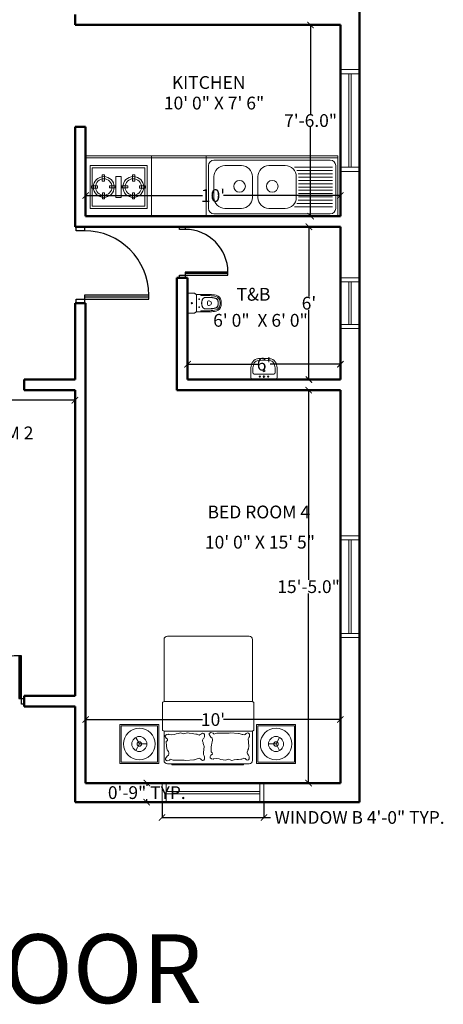
# Model space of a CAD drawing. Units: inches. Extents: x 147 to 1638, y 107 to 941.
# Tile 9 of 17: x 542 to 741, y 107 to 570. Entities that reach past the tile are written whole.
import ezdxf

# ---------------------------------------------------------------- set-up
doc = ezdxf.new("R2010")
doc.units = ezdxf.units.IN
doc.header["$MEASUREMENT"] = 0
for name, color, linetype, lineweight in [('A-ANNO-DIMS', 2, 'Continuous', 15), ('A-ANNO-TEXT', 7, 'Continuous', 25), ('A-AREA-IDEN', 7, 'Continuous', 18), ('A-Door', 150, 'Continuous', 25), ('A-EQPM', 8, 'Continuous', 18), ('A-FLOR-CASE', 9, 'Continuous', 20), ('A-FLOR-FIXT', 9, 'Continuous', 18), ('furniture', 50, 'Continuous', 18), ('walls', 7, 'Continuous', 50), ('windows', 3, 'Continuous', 20)]:
    doc.layers.add(name, color=color, linetype=linetype, lineweight=lineweight)
doc.layers.add('A-Glaz', color=92, linetype='Continuous')
doc.layers.add('NT', color=1, linetype='Continuous')
doc.styles.get("Standard").update_dxf_attribs({"font": 'arial.ttf'})
doc.dimstyles.get("Standard").update_dxf_attribs({"dimtxt": 6, "dimasz": 3, "dimexe": 0.18, "dimexo": 0.0625, "dimgap": 0.09, "dimtad": 0, "dimtih": 1, "dimtoh": 1, "dimdec": 1, "dimzin": 0, "dimdsep": 46, "dimlunit": 3, "dimtxsty": 'Standard', "dimblk": 'ARCHTICK', "dimcen": 0.09, "dimadec": 0, "dimazin": 0, "dimtfac": 1, "dimtdec": 1, "dimtofl": 0, "dimtmove": 0, "dimatfit": 3, "dimfxl": 1, "dimtolj": 1, "dimtzin": 0, "dimarcsym": 0})

# ---------------------------------------------------------------- blocks, each defined once
blk = doc.blocks.new('A$C087A3AA9')
at = {"layer": 'A-Door'}
for points in [[(853, 95), (853, 853), (805, 853), (805, 95)], [(47, 95), (47, 0), (0, 0), (0, 95)], [(900, 95), (900, 0), (853, 0), (853, 95)]]:
    blk.add_lwpolyline(points, close=True, dxfattribs=at)
at = {"layer": 'A-Glaz'}
blk.add_line((829, 853), (829, 95), dxfattribs=at)
at = {"layer": 'NT'}
blk.add_arc((805, 95), 758, 90, 180, dxfattribs=at)
blk = doc.blocks.new('_ArchTick')
at = {"color": 0, "linetype": 'ByBlock', "const_width": 0.15}
blk.add_lwpolyline([(-0.5, -0.5), (0.5, 0.5)], dxfattribs=at)
blk = doc.blocks.new('*D18')
at = {"layer": 'A-ANNO-DIMS', "color": 0, "lineweight": -2, "transparency": 16777216}
for p, q in [((620.94, 408.03), (620.94, 408.14)), ((692.94, 408.03), (692.94, 408.14)), ((620.94, 407.96), (654.08, 407.96)), ((692.94, 407.96), (659.81, 407.96))]:
    blk.add_line(p, q, dxfattribs=at)
at = {"layer": 'Defpoints', "color": 0, "lineweight": -2, "transparency": 16777216}
for p in [(620.94, 407.96), (692.94, 407.96), (692.94, 407.96)]:
    blk.add_point(p, dxfattribs=at)
at = {"layer": 'A-ANNO-DIMS', "color": 0, "lineweight": -2, "transparency": 16777216, "xscale": 3, "yscale": 3, "zscale": 3, "rotation": 180}
blk.add_blockref('_ArchTick', (620.94, 407.96), dxfattribs=at)
at = {"layer": 'A-ANNO-DIMS', "color": 0, "lineweight": -2, "transparency": 16777216, "xscale": 3, "yscale": 3, "zscale": 3}
blk.add_blockref('_ArchTick', (692.94, 407.96), dxfattribs=at)
at = {"layer": 'A-ANNO-DIMS', "color": 0, "transparency": 16777216, "insert": (656.94, 407.96), "char_height": 6, "attachment_point": 5}
blk.add_mtext("\\A1;6'", dxfattribs=at)
blk = doc.blocks.new('*D19')
at = {"layer": 'A-ANNO-DIMS', "color": 0, "lineweight": -2, "transparency": 16777216}
for p, q in [((678.55, 472.72), (677.93, 472.72)), ((678.11, 472.72), (678.11, 439.87)), ((678.11, 400.72), (678.11, 433.56)), ((678.55, 400.72), (677.93, 400.72))]:
    blk.add_line(p, q, dxfattribs=at)
at = {"layer": 'Defpoints', "color": 0, "lineweight": -2, "transparency": 16777216}
for p in [(678.61, 472.72), (678.11, 400.72), (678.61, 400.72)]:
    blk.add_point(p, dxfattribs=at)
at = {"layer": 'A-ANNO-DIMS', "color": 0, "lineweight": -2, "transparency": 16777216, "xscale": 3, "yscale": 3, "zscale": 3}
for p, rotation in [((678.11, 472.72), 90), ((678.11, 400.72), 270)]:
    blk.add_blockref('_ArchTick', p, dxfattribs=dict(at, rotation=rotation))
at = {"layer": 'A-ANNO-DIMS', "color": 0, "transparency": 16777216, "insert": (678.11, 436.72), "char_height": 6, "attachment_point": 5}
blk.add_mtext("\\A1;6'", dxfattribs=at)
blk = doc.blocks.new('*D20')
at = {"layer": 'A-ANNO-DIMS', "color": 0, "lineweight": -2, "transparency": 16777216}
for p, q in [((665.57, 567.72), (679.08, 567.72)), ((678.9, 567.72), (678.9, 525.87)), ((678.9, 477.72), (678.9, 519.56)), ((665.57, 477.72), (679.08, 477.72))]:
    blk.add_line(p, q, dxfattribs=at)
at = {"layer": 'Defpoints', "color": 0, "lineweight": -2, "transparency": 16777216}
for p in [(665.51, 567.72), (665.51, 477.72), (678.9, 477.72)]:
    blk.add_point(p, dxfattribs=at)
at = {"layer": 'A-ANNO-DIMS', "color": 0, "lineweight": -2, "transparency": 16777216, "xscale": 3, "yscale": 3, "zscale": 3}
for p, rotation in [((678.9, 567.72), 90), ((678.9, 477.72), 270)]:
    blk.add_blockref('_ArchTick', p, dxfattribs=dict(at, rotation=rotation))
at = {"layer": 'A-ANNO-DIMS', "color": 0, "transparency": 16777216, "insert": (678.9, 522.72), "char_height": 6, "attachment_point": 5}
blk.add_mtext('\\A1;7\'-6.0"', dxfattribs=at)
blk = doc.blocks.new('*D21')
at = {"layer": 'A-ANNO-DIMS', "color": 0, "lineweight": -2, "transparency": 16777216}
for p, q in [((572.94, 484.18), (572.94, 487.58)), ((572.94, 487.4), (628.05, 487.4)), ((692.94, 487.4), (637.84, 487.4)), ((692.94, 484.18), (692.94, 487.58))]:
    blk.add_line(p, q, dxfattribs=at)
at = {"layer": 'Defpoints', "color": 0, "lineweight": -2, "transparency": 16777216}
for p in [(692.94, 487.4), (572.94, 484.12), (692.94, 484.12)]:
    blk.add_point(p, dxfattribs=at)
at = {"layer": 'A-ANNO-DIMS', "color": 0, "lineweight": -2, "transparency": 16777216, "xscale": 3, "yscale": 3, "zscale": 3, "rotation": 180}
blk.add_blockref('_ArchTick', (572.94, 487.4), dxfattribs=at)
at = {"layer": 'A-ANNO-DIMS', "color": 0, "lineweight": -2, "transparency": 16777216, "xscale": 3, "yscale": 3, "zscale": 3}
blk.add_blockref('_ArchTick', (692.94, 487.4), dxfattribs=at)
at = {"layer": 'A-ANNO-DIMS', "color": 0, "transparency": 16777216, "insert": (632.94, 487.4), "char_height": 6, "attachment_point": 5}
blk.add_mtext("\\A1;10'", dxfattribs=at)
blk = doc.blocks.new('*D22')
at = {"layer": 'A-ANNO-DIMS', "color": 0, "lineweight": -2, "transparency": 16777216}
for p, q in [((572.94, 231.3), (572.94, 240.81)), ((572.94, 240.63), (628.05, 240.63)), ((692.94, 240.63), (637.84, 240.63)), ((692.94, 231.3), (692.94, 240.81))]:
    blk.add_line(p, q, dxfattribs=at)
at = {"layer": 'Defpoints', "color": 0, "lineweight": -2, "transparency": 16777216}
for p in [(692.94, 240.63), (572.94, 231.24), (692.94, 231.24)]:
    blk.add_point(p, dxfattribs=at)
at = {"layer": 'A-ANNO-DIMS', "color": 0, "lineweight": -2, "transparency": 16777216, "xscale": 3, "yscale": 3, "zscale": 3, "rotation": 180}
blk.add_blockref('_ArchTick', (572.94, 240.63), dxfattribs=at)
at = {"layer": 'A-ANNO-DIMS', "color": 0, "lineweight": -2, "transparency": 16777216, "xscale": 3, "yscale": 3, "zscale": 3}
blk.add_blockref('_ArchTick', (692.94, 240.63), dxfattribs=at)
at = {"layer": 'A-ANNO-DIMS', "color": 0, "transparency": 16777216, "insert": (632.94, 240.63), "char_height": 6, "attachment_point": 5}
blk.add_mtext("\\A1;10'", dxfattribs=at)
blk = doc.blocks.new('*D23')
at = {"layer": 'A-ANNO-DIMS', "color": 0, "lineweight": -2, "transparency": 16777216}
for p, q in [((684.27, 395.72), (677.76, 395.72)), ((677.94, 395.72), (677.94, 306.37)), ((677.94, 210.72), (677.94, 300.06)), ((684.27, 210.72), (677.76, 210.72))]:
    blk.add_line(p, q, dxfattribs=at)
at = {"layer": 'Defpoints', "color": 0, "lineweight": -2, "transparency": 16777216}
for p in [(684.33, 395.72), (677.94, 210.72), (684.33, 210.72)]:
    blk.add_point(p, dxfattribs=at)
at = {"layer": 'A-ANNO-DIMS', "color": 0, "lineweight": -2, "transparency": 16777216, "xscale": 3, "yscale": 3, "zscale": 3}
for p, rotation in [((677.94, 395.72), 90), ((677.94, 210.72), 270)]:
    blk.add_blockref('_ArchTick', p, dxfattribs=dict(at, rotation=rotation))
at = {"layer": 'A-ANNO-DIMS', "color": 0, "transparency": 16777216, "insert": (677.94, 303.22), "char_height": 6, "attachment_point": 5}
blk.add_mtext('\\A1;15\'-5.0"', dxfattribs=at)
blk = doc.blocks.new('*D29')
at = {"layer": 'A-ANNO-DIMS', "color": 0, "lineweight": -2, "transparency": 16777216}
for p, q in [((471.94, 391.04), (471.94, 391.15)), ((471.94, 390.97), (517.09, 390.97)), ((567.94, 390.97), (522.8, 390.97)), ((567.94, 391.04), (567.94, 391.15))]:
    blk.add_line(p, q, dxfattribs=at)
at = {"layer": 'Defpoints', "color": 0, "lineweight": -2, "transparency": 16777216}
for p in [(471.94, 390.97), (567.94, 390.97), (567.94, 390.97)]:
    blk.add_point(p, dxfattribs=at)
at = {"layer": 'A-ANNO-DIMS', "color": 0, "lineweight": -2, "transparency": 16777216, "xscale": 3, "yscale": 3, "zscale": 3, "rotation": 180}
blk.add_blockref('_ArchTick', (471.94, 390.97), dxfattribs=at)
at = {"layer": 'A-ANNO-DIMS', "color": 0, "lineweight": -2, "transparency": 16777216, "xscale": 3, "yscale": 3, "zscale": 3}
blk.add_blockref('_ArchTick', (567.94, 390.97), dxfattribs=at)
at = {"layer": 'A-ANNO-DIMS', "color": 0, "transparency": 16777216, "insert": (519.94, 390.97), "char_height": 6, "attachment_point": 5}
blk.add_mtext("\\A1;8'", dxfattribs=at)
blk = doc.blocks.new('MAT-P14')
for p, q in [((-1.337, 1.348), (-1.337, 1.948)), ((-1.337, 1.948), (-0.737, 1.948)), ((-1.317, 1.928), (-0.757, 1.928)), ((-1.317, 1.368), (-1.317, 1.928)), ((-0.757, 1.368), (-0.757, 1.928)), ((-0.737, 1.348), (-0.737, 1.948)), ((0.625, 1.95), (-0.625, 1.95)), ((0.753, 1.348), (0.753, 1.948)), ((1.353, 1.948), (0.753, 1.948)), ((1.333, 1.928), (0.773, 1.928)), ((0.773, 1.368), (0.773, 1.928)), ((1.333, 1.368), (1.333, 1.928)), ((1.353, 1.348), (1.353, 1.948)), ((-1.037, 1.648), (-1.091, 1.749)), ((1.053, 1.648), (1.108, 1.749)), ((-1.037, 1.648), (-1.091, 1.547)), ((-1.037, 1.648), (-0.922, 1.648)), ((1.053, 1.648), (0.938, 1.648)), ((1.053, 1.648), (1.108, 1.547)), ((-1.317, 1.368), (-0.757, 1.368)), ((1.333, 1.368), (0.773, 1.368)), ((-1.337, 1.348), (-0.737, 1.348)), ((1.353, 1.348), (0.753, 1.348))]:
    blk.add_line(p, q)
blk.add_lwpolyline([(-0.542, 1.95), (-0.542, 1.967), (0.558, 1.967), (0.558, 1.95)], close=True)
for points in [[(-0.675, 1.45), (-0.675, 1.9, -0.414214), (-0.625, 1.95), (0.625, 1.95, -0.414214), (0.675, 1.9), (0.675, 1.45)], [(-0.675, 1, -0.414214), (-0.7, 1.025), (-0.7, 1.425, -0.414214), (-0.675, 1.45), (0.675, 1.45, -0.414214), (0.7, 1.425), (0.7, 1.025, -0.414214), (0.675, 1)], [(-0.625, 0, -0.414214), (-0.675, 0.05), (-0.675, 1), (0.675, 1), (0.675, 0.05, -0.414214), (0.625, 0)]]:
    blk.add_lwpolyline(points, format="xyb", close=True)
for points in [[(-0.614, 1.818), (-0.626, 1.838), (-0.626, 1.877), (-0.614, 1.891), (-0.596, 1.896), (-0.579, 1.886), (-0.563, 1.872), (-0.545, 1.863), (-0.516, 1.879), (-0.497, 1.882), (-0.465, 1.884), (-0.439, 1.887), (-0.395, 1.892), (-0.363, 1.9), (-0.309, 1.882), (-0.262, 1.897), (-0.23, 1.892), (-0.192, 1.884), (-0.166, 1.873), (-0.128, 1.868), (-0.082, 1.875), (-0.076, 1.88), (-0.052, 1.875), (-0.028, 1.861), (-0.028, 1.841), (-0.04, 1.817), (-0.064, 1.802), (-0.06, 1.781), (-0.043, 1.768), (-0.046, 1.697), (-0.05, 1.662), (-0.056, 1.64), (-0.062, 1.612), (-0.068, 1.596), (-0.068, 1.579), (-0.063, 1.56), (-0.039, 1.545), (-0.015, 1.505), (-0.015, 1.486), (-0.038, 1.471), (-0.075, 1.482), (-0.081, 1.487), (-0.087, 1.497), (-0.134, 1.481), (-0.304, 1.482), (-0.318, 1.482), (-0.335, 1.479), (-0.464, 1.488), (-0.467, 1.486), (-0.473, 1.486), (-0.517, 1.503), (-0.53, 1.505), (-0.548, 1.51), (-0.566, 1.501), (-0.581, 1.487), (-0.599, 1.477), (-0.617, 1.482), (-0.629, 1.497), (-0.629, 1.536), (-0.623, 1.55), (-0.611, 1.57), (-0.614, 1.614), (-0.615, 1.627), (-0.618, 1.644), (-0.619, 1.66), (-0.62, 1.675), (-0.62, 1.695), (-0.618, 1.707), (-0.614, 1.723), (-0.608, 1.739), (-0.604, 1.75), (-0.598, 1.771), (-0.596, 1.785), (-0.6, 1.798), (-0.614, 1.819)], [(0.069, 1.559), (0.057, 1.54), (0.057, 1.501), (0.069, 1.486), (0.087, 1.481), (0.105, 1.491), (0.121, 1.505), (0.139, 1.514), (0.168, 1.498), (0.187, 1.496), (0.219, 1.493), (0.244, 1.49), (0.289, 1.485), (0.321, 1.477), (0.374, 1.495), (0.422, 1.48), (0.454, 1.486), (0.492, 1.493), (0.517, 1.504), (0.555, 1.509), (0.602, 1.502), (0.608, 1.497), (0.632, 1.502), (0.656, 1.517), (0.656, 1.536), (0.644, 1.561), (0.62, 1.575), (0.624, 1.596), (0.641, 1.609), (0.637, 1.68), (0.633, 1.715), (0.628, 1.738), (0.606, 1.765), (0.6, 1.781), (0.6, 1.798), (0.605, 1.817), (0.629, 1.832), (0.654, 1.872), (0.654, 1.892), (0.63, 1.906), (0.593, 1.895), (0.587, 1.891), (0.581, 1.881), (0.534, 1.896), (0.379, 1.896), (0.366, 1.896), (0.348, 1.898), (0.22, 1.89), (0.216, 1.891), (0.21, 1.891), (0.167, 1.875), (0.154, 1.872), (0.136, 1.867), (0.118, 1.876), (0.102, 1.89), (0.085, 1.9), (0.067, 1.895), (0.055, 1.881), (0.055, 1.842), (0.061, 1.827), (0.073, 1.807), (0.07, 1.764), (0.069, 1.75), (0.066, 1.733), (0.065, 1.718), (0.063, 1.703), (0.063, 1.682), (0.066, 1.67), (0.07, 1.655), (0.075, 1.638), (0.079, 1.627), (0.086, 1.607), (0.087, 1.592), (0.083, 1.579), (0.07, 1.559)]]:
    blk.add_lwpolyline(points)
for centre, radius in [((-1.037, 1.648), 0.24), ((1.053, 1.648), 0.24), ((-1.037, 1.648), 0.115), ((-1.037, 1.648), 0.035), ((1.053, 1.648), 0.115), ((1.053, 1.648), 0.035)]:
    blk.add_circle(centre, radius)
blk = doc.blocks.new('2SAINDA')
at = {"color": 0, "linetype": 'ByBlock'}
for p, q in [((0.018, 0.2), (0.141, 0.2)), ((0, 0.188), (0, -0.188)), ((0.157, 0.192), (0.162, 0.188)), ((0.18, -0.164), (0.18, 0.164)), ((0.279, 0.159), (0.261, 0.176)), ((0.437, 0.047), (0.424, 0.047)), ((0.157, -0.192), (0.162, -0.188)), ((0.279, -0.159), (0.261, -0.176)), ((0.437, -0.047), (0.424, -0.047)), ((0.018, -0.2), (0.141, -0.2))]:
    blk.add_line(p, q, dxfattribs=at)
for centre, radius in [((0.09, 0), 0.0135), ((0.09, 0), 0.0135), ((0.236, 0.08), 0.0075), ((0.236, -0.08), 0.0075)]:
    blk.add_circle(centre, radius, dxfattribs=at)
for centre, radius, start, end in [((0.018, 0.18), 0.02, 90, 155.6901), ((0.141, 0.181), 0.019, 34.9372, 90), ((0.155, 0.164), 0.025, 23.3776, 73.7848), ((0.383, -5.322), 5.5, 89.2905, 92.1362), ((0.155, 0.164), 0.025, 360, 23.3776), ((0.293, 0.173), 0.02, 225, 270.9364), ((0.485, 0), 0.2, 160.016, 199.984), ((0.485, 0), 0.196, 160.016, 199.984), ((0.383, -5.322), 5.476, 89.2905, 90.9364), ((0.368, 0.043), 0.075, 90.1648, 160.016), ((0.368, 0.043), 0.071, 90.1648, 160.016), ((0.383, -5.322), 5.44, 89.2905, 90.1648), ((0.383, -5.322), 5.436, 89.2905, 90.1648), ((0.582, 0), 0.18, 170.2849, 189.7151), ((0.424, 0.027), 0.02, 90, 170.2849), ((0.437, 0), 0.047, 0, 90), ((0.437, 0), 0.047, 270, 0), ((0.444, -0.373), 0.49, 75.4605, 89.2905), ((0.444, -0.373), 0.486, 75.4605, 89.2905), ((0.444, -0.373), 0.55, 75.4605, 89.2905), ((0.444, -0.373), 0.526, 75.4605, 89.2905), ((0.549, 0.03), 0.07, 8.8162, 75.4605), ((0.549, 0.03), 0.074, 8.8162, 75.4605), ((0.549, 0.03), 0.11, 8.8162, 75.4605), ((0.549, 0.03), 0.134, 8.8162, 75.4605), ((0.355, 0), 0.266, 351.1838, 8.8162), ((0.355, 0), 0.27, 351.1838, 8.8162), ((0.355, 0), 0.306, 351.1838, 8.8162), ((0.355, 0), 0.33, 351.1838, 8.8162), ((0.018, -0.18), 0.02, 204.3099, 270), ((0.141, -0.181), 0.019, 270, 325.0628), ((0.155, -0.164), 0.025, 286.2152, 336.6224), ((0.155, -0.164), 0.025, 336.6224, 0), ((0.383, 5.322), 5.5, 267.8638, 270.7095), ((0.293, -0.173), 0.02, 89.0636, 135), ((0.383, 5.322), 5.476, 269.0636, 270.7095), ((0.368, -0.043), 0.075, 199.984, 269.8352), ((0.368, -0.043), 0.071, 199.984, 269.8352), ((0.383, 5.322), 5.436, 269.8352, 270.7095), ((0.383, 5.322), 5.44, 269.8352, 270.7095), ((0.424, -0.027), 0.02, 189.7151, 270), ((0.444, 0.373), 0.486, 270.7095, 284.5395), ((0.444, 0.373), 0.49, 270.7095, 284.5395), ((0.444, 0.373), 0.526, 270.7095, 284.5395), ((0.444, 0.373), 0.55, 270.7095, 284.5395), ((0.549, -0.03), 0.07, 284.5395, 351.1838), ((0.549, -0.03), 0.074, 284.5395, 351.1838), ((0.549, -0.03), 0.11, 284.5395, 351.1838), ((0.549, -0.03), 0.134, 284.5395, 351.1838)]:
    blk.add_arc(centre, radius, start, end, dxfattribs=at)
blk = doc.blocks.new('2SALADA2')
at = {"color": 0}
for p, q in [((-0.296, 0), (0.296, 0)), ((0.207, -0.13), (-0.207, -0.13))]:
    blk.add_line(p, q, dxfattribs=at)
for centre, radius in [((-0.1, -0.07), 0.015), ((0, -0.205), 0.023), ((0, -0.07), 0.0175), ((0.1, -0.07), 0.015)]:
    blk.add_circle(centre, radius, dxfattribs=at)
for centre, radius, start, end in [((-0.296, -0.01), 0.01, 90, 173.6262), ((0.296, -0.01), 0.01, 6.3738, 90), ((1.185, -0.175), 1.5, 173.6262, 182.693), ((1.186, -0.221), 1.454, 178.0234, 180.898), ((-0.227, -0.171), 0.04, 95.5937, 179.6995), ((-0.207, -0.38), 0.25, 90, 95.5937), ((0.207, -0.38), 0.25, 84.4063, 90), ((0.227, -0.171), 0.04, 0.3005, 84.4063), ((-1.186, -0.221), 1.454, 359.102, 1.9766), ((-1.185, -0.175), 1.5, 357.307, 6.3738), ((0.186, -0.222), 0.5, 182.693, 199.3406), ((-0.135, -0.335), 0.16, 199.3406, 257.4429), ((0.186, -0.222), 0.454, 182.693, 199.3406), ((-0.135, -0.335), 0.114, 199.3406, 257.4429), ((-0.061, -0.003), 0.454, 257.4429, 266.4982), ((0, 0.995), 1.454, 266.4982, 273.5018), ((0.061, -0.003), 0.454, 273.5018, 282.5571), ((0.135, -0.335), 0.114, 282.5571, 340.6594), ((0.135, -0.335), 0.16, 282.5571, 340.6594), ((-0.186, -0.222), 0.454, 340.6594, 357.307), ((-0.186, -0.222), 0.5, 340.6594, 357.307), ((-0.061, -0.003), 0.5, 257.4429, 266.4982), ((0, 0.995), 1.5, 266.4982, 273.5018), ((0.061, -0.003), 0.5, 273.5018, 282.5571)]:
    blk.add_arc(centre, radius, start, end, dxfattribs=at)
blk = doc.blocks.new('WIN-48IN')
for p, q in [((9, 48), (0, 48)), ((0, 48), (0, 0)), ((9, 0), (9, 48)), ((9, 46), (0, 46)), ((4, 2), (4, 46)), ((5, 2), (5, 46)), ((0, 2), (9, 2)), ((0, 0), (9, 0))]:
    blk.add_line(p, q)
blk = doc.blocks.new('WIN-24IN')
for p, q in [((9, 24), (0, 24)), ((0, 24), (0, 0)), ((9, 0), (9, 24)), ((9, 22), (0, 22)), ((4, 2), (4, 22)), ((5, 2), (5, 22)), ((0, 2), (9, 2)), ((0, 0), (9, 0))]:
    blk.add_line(p, q)
blk = doc.blocks.new('CABINET-KITCHEN-RUN')
for p, q in [((0, 28.41), (118.8, 28.41)), ((0, 0), (0, 28.41)), ((30.99, 0), (30.99, 28.41)), ((56.82, 0), (56.82, 28.41)), ((118.8, 28.41), (118.8, 0)), ((0, 27.38), (118.8, 27.38)), ((118.8, 0), (0, 0))]:
    blk.add_line(p, q)
blk = doc.blocks.new('COOKTOP-2-BURNER')
for p, q in [((0, 0), (0, 20.15)), ((0, 20.15), (26.86, 20.15)), ((1.03, 1.03), (1.03, 19.11)), ((1.03, 19.11), (25.83, 19.11)), ((25.83, 1.03), (25.83, 19.11)), ((26.86, 0), (26.86, 20.15)), ((5.75, 15.75), (5.75, 12.91)), ((5.75, 15.75), (6.79, 15.75)), ((6.79, 15.75), (6.79, 12.91)), ((12.14, 14.98), (14.72, 14.98)), ((12.14, 14.98), (12.14, 5.17)), ((14.72, 14.98), (14.72, 5.17)), ((21.11, 15.75), (20.07, 15.75)), ((20.07, 15.75), (20.07, 12.91)), ((21.11, 15.75), (21.11, 12.91)), ((0.69, 9.55), (0.69, 10.59)), ((0.69, 10.59), (3.53, 10.59)), ((0.69, 9.55), (3.53, 9.55)), ((3.53, 9.55), (3.53, 10.59)), ((5.75, 12.91), (6.79, 12.91)), ((11.95, 10.69), (9.11, 10.69)), ((9.11, 10.69), (9.11, 9.66)), ((11.95, 9.66), (9.11, 9.66)), ((11.95, 10.69), (11.95, 9.66)), ((14.91, 10.69), (17.75, 10.69)), ((14.91, 10.69), (14.91, 9.66)), ((14.91, 9.66), (17.75, 9.66)), ((17.75, 10.69), (17.75, 9.66)), ((21.11, 12.91), (20.07, 12.91)), ((23.33, 9.55), (23.33, 10.59)), ((26.17, 10.59), (23.33, 10.59)), ((26.17, 9.55), (23.33, 9.55)), ((26.17, 9.55), (26.17, 10.59)), ((5.86, 4.49), (5.86, 7.33)), ((6.89, 7.33), (5.86, 7.33)), ((6.89, 4.49), (6.89, 7.33)), ((12.14, 5.17), (14.72, 5.17)), ((19.97, 4.49), (19.97, 7.33)), ((19.97, 7.33), (21, 7.33)), ((21, 4.49), (21, 7.33)), ((0, 0), (26.86, 0)), ((1.03, 1.03), (25.83, 1.03)), ((6.89, 4.49), (5.86, 4.49)), ((19.97, 4.49), (21, 4.49))]:
    blk.add_line(p, q)
for centre, radius in [((6.48, 10.08), 4.91), ((6.48, 10.08), 3.87), ((20.38, 10.08), 4.91), ((20.38, 10.08), 3.87)]:
    blk.add_circle(centre, radius)
blk = doc.blocks.new('SINK-DOUBLE-DRAINBOARD')
for p, q in [((57.34, 25.31), (2.58, 25.31)), ((0, 22.73), (0, 2.58)), ((15.5, 22.73), (7.75, 22.73)), ((36.16, 22.73), (28.41, 22.73)), ((40.53, 21.95), (58.37, 21.95)), ((41.67, 20.4), (58.37, 20.4)), ((42.22, 18.85), (58.37, 18.85)), ((59.92, 2.58), (59.92, 22.73)), ((2.58, 17.56), (2.58, 7.75)), ((20.66, 17.56), (20.66, 7.75)), ((23.24, 17.56), (23.24, 7.75)), ((41.32, 17.56), (41.32, 7.75)), ((42.36, 17.3), (58.37, 17.3)), ((42.36, 15.75), (58.37, 15.75)), ((42.36, 14.2), (58.37, 14.2)), ((42.36, 12.66), (58.37, 12.66)), ((42.36, 11.11), (58.37, 11.11)), ((42.36, 9.56), (58.37, 9.56)), ((41.67, 4.91), (58.37, 4.91)), ((42.22, 6.46), (58.37, 6.46)), ((42.36, 8.01), (58.37, 8.01)), ((2.58, 0), (57.34, 0)), ((7.75, 2.58), (15.5, 2.58)), ((28.41, 2.58), (36.16, 2.58)), ((40.53, 3.36), (58.37, 3.36))]:
    blk.add_line(p, q)
for centre in [(14.61, 13), (30.02, 13)]:
    blk.add_circle(centre, 2.75)
for centre, radius, start, end in [((2.58, 22.73), 2.58, 90, 180), ((57.34, 22.73), 2.58, 0, 90), ((7.75, 17.56), 5.17, 90, 180), ((15.5, 17.56), 5.17, 0, 90), ((28.41, 17.56), 5.17, 90, 180), ((36.16, 17.56), 5.17, 0, 90), ((7.75, 7.75), 5.17, 180, 270), ((15.5, 7.75), 5.17, 270, 0), ((28.41, 7.75), 5.17, 180, 270), ((36.16, 7.75), 5.17, 270, 0), ((2.58, 2.58), 2.58, 180, 270), ((57.34, 2.58), 2.58, 270, 0)]:
    blk.add_arc(centre, radius, start, end)
blk = doc.blocks.new('*D104')
at = {"layer": 'A-ANNO-DIMS', "color": 0, "lineweight": -2, "transparency": 16777216}
for p, q in [((608.94, 201.66), (608.94, 194.34)), ((656.94, 201.66), (656.94, 194.34)), ((608.94, 194.52), (656.94, 194.52)), ((656.94, 194.52), (659.94, 194.52))]:
    blk.add_line(p, q, dxfattribs=at)
at = {"layer": 'Defpoints', "color": 0, "lineweight": -2, "transparency": 16777216}
for p in [(608.94, 201.72), (656.94, 201.72), (656.94, 194.52)]:
    blk.add_point(p, dxfattribs=at)
at = {"layer": 'A-ANNO-DIMS', "color": 0, "lineweight": -2, "transparency": 16777216, "xscale": 3, "yscale": 3, "zscale": 3, "rotation": 180}
blk.add_blockref('_ArchTick', (608.94, 194.52), dxfattribs=at)
at = {"layer": 'A-ANNO-DIMS', "color": 0, "lineweight": -2, "transparency": 16777216, "xscale": 3, "yscale": 3, "zscale": 3}
blk.add_blockref('_ArchTick', (656.94, 194.52), dxfattribs=at)
at = {"layer": 'A-ANNO-DIMS', "color": 0, "transparency": 16777216, "insert": (701.96, 194.52), "char_height": 6, "attachment_point": 5}
blk.add_mtext('\\A1;WINDOW B 4\'-0" TYP.', dxfattribs=at)
blk = doc.blocks.new('*D105')
at = {"layer": 'A-ANNO-DIMS', "color": 0, "lineweight": -2, "transparency": 16777216}
for p, q in [((608.88, 210.72), (601.56, 210.72)), ((601.74, 210.72), (601.74, 209.37)), ((608.88, 201.72), (601.56, 201.72)), ((601.74, 201.72), (601.74, 203.06))]:
    blk.add_line(p, q, dxfattribs=at)
at = {"layer": 'Defpoints', "color": 0, "lineweight": -2, "transparency": 16777216}
for p in [(608.94, 210.72), (601.74, 201.72), (608.94, 201.72)]:
    blk.add_point(p, dxfattribs=at)
at = {"layer": 'A-ANNO-DIMS', "color": 0, "lineweight": -2, "transparency": 16777216, "xscale": 3, "yscale": 3, "zscale": 3}
for p, rotation in [((601.74, 210.72), 90), ((601.74, 201.72), 270)]:
    blk.add_blockref('_ArchTick', p, dxfattribs=dict(at, rotation=rotation))
at = {"layer": 'A-ANNO-DIMS', "color": 0, "transparency": 16777216, "insert": (601.74, 206.22), "char_height": 6, "attachment_point": 5}
blk.add_mtext('\\A1;0\'-9" TYP.', dxfattribs=at)

msp = doc.modelspace()

# ---------------------------------------------------------------- linework, layer by layer
at = {"layer": 'walls'}
for p, q in [((701.94, 909.72), (701.94, 201.72)), ((567.94, 572.72), (567.94, 567.72)), ((572.94, 567.72), (567.94, 567.72)), ((572.94, 567.72), (692.94, 567.72)), ((692.94, 567.72), (692.94, 477.72)), ((567.94, 519.72), (567.94, 472.72)), ((572.94, 519.72), (567.94, 519.72)), ((572.94, 519.72), (572.94, 477.72)), ((572.94, 477.72), (692.94, 477.72)), ((572.94, 472.72), (567.94, 472.72)), ((572.94, 472.72), (615.94, 472.72)), ((615.94, 472.72), (620.94, 472.72)), ((620.94, 472.72), (692.94, 472.72)), ((692.94, 472.72), (692.94, 400.72)), ((615.94, 448.72), (615.94, 395.72)), ((615.94, 448.72), (620.94, 448.72)), ((620.94, 448.72), (620.94, 400.72)), ((567.94, 436.72), (567.94, 400.72)), ((572.94, 436.72), (567.94, 436.72)), ((572.94, 436.72), (572.94, 210.72)), ((543.94, 400.72), (543.94, 395.72)), ((543.94, 400.72), (567.94, 400.72)), ((620.94, 400.72), (692.94, 400.72)), ((543.94, 395.72), (567.94, 395.72)), ((567.94, 395.72), (567.94, 251.72)), ((615.94, 395.72), (692.94, 395.72)), ((692.94, 395.72), (692.94, 210.72)), ((543.94, 251.72), (543.94, 246.72)), ((543.94, 251.72), (567.94, 251.72)), ((543.94, 246.72), (567.94, 246.72)), ((567.94, 246.72), (567.94, 201.72)), ((572.94, 210.72), (692.94, 210.72)), ((567.94, 201.72), (701.94, 201.72))]:
    msp.add_line(p, q, dxfattribs=at)

# ---------------------------------------------------------------- block references
at = {"layer": 'A-Door', "rotation": 270}
for p, xscale, yscale, zscale in [((568.55, 472.72), 0.0400000000000001, 0.0400000000000001, 0.0400000000000001), ((617.21, 472.72), 0.0266666667542921, 0.0266666667542921, 0.0266666667542921)]:
    msp.add_blockref('A$C087A3AA9', p, dxfattribs=dict(at, xscale=xscale, yscale=yscale, zscale=zscale))
at = {"layer": 'A-Door', "xscale": 0.0266666667542921, "yscale": 0.0266666667542921, "zscale": 0.0266666667542921}
msp.add_blockref('A$C087A3AA9', (519.94, 247.95), dxfattribs=at)
at = {"layer": 'A-EQPM'}
msp.add_blockref('COOKTOP-2-BURNER', (575.01, 481.33), dxfattribs=at)
at = {"layer": 'A-FLOR-CASE'}
msp.add_blockref('CABINET-KITCHEN-RUN', (572.94, 477.72), dxfattribs=at)
at = {"layer": 'A-FLOR-FIXT'}
msp.add_blockref('SINK-DOUBLE-DRAINBOARD', (630.8, 478.75), dxfattribs=at)
at = {"layer": 'A-FLOR-FIXT', "xscale": 23.19012112898009, "yscale": 23.19012112898009, "zscale": 23.19012112898009}
msp.add_blockref('2SAINDA', (620.94, 436.72), dxfattribs=at)
at = {"layer": 'A-FLOR-FIXT', "xscale": 19.81841434140962, "yscale": 19.81841434140962, "zscale": 19.81841434140962, "rotation": 180}
msp.add_blockref('2SALADA2', (656.94, 400.72), dxfattribs=at)
at = {"layer": 'furniture', "xscale": 30.80045642108221, "yscale": 30.80045642108221, "zscale": 30.80045642108221, "rotation": 180}
msp.add_blockref('MAT-P14', (630.67, 279.88), dxfattribs=at)
at = {"layer": 'windows'}
for name, p in [('WIN-48IN', (692.94, 498.72)), ('WIN-24IN', (692.94, 424.72)), ('WIN-48IN', (692.94, 279.22))]:
    msp.add_blockref(name, p, dxfattribs=at)
at = {"layer": 'windows', "rotation": 270.0000000000001}
msp.add_blockref('WIN-48IN', (608.94, 210.72), dxfattribs=at)

# ---------------------------------------------------------------- texts
at = {"layer": 'A-ANNO-TEXT'}
msp.add_text('GROUND FLOOR', height=32.387, dxfattribs=at).set_placement((290.4, 107.1))
at = {"layer": 'A-AREA-IDEN'}
for s, height, p in [('KITCHEN ', 6.031, (613.54, 537.63)), ('  10\' 0" X 7\' 6"', 6.0306, (606.09, 527.94)), ('T&B', 6.031, (644.04, 437.89)), ('  6\' 0"  X 6\' 0"', 6.0306, (629.32, 425.62)), ('LIVING ROOM 2', 6.0306, (490.37, 372.59)), ('BED ROOM 4', 6.031, (630.35, 335.37)), ('  10\' 0" X 15\' 5"', 6.0306, (625.42, 321.14))]:
    msp.add_text(s, height=height, dxfattribs=at).set_placement(p)

# ---------------------------------------------------------------- dimensions: what is measured, and where the dimension line sits
at = {"layer": 'A-ANNO-DIMS'}
for base, p1, p2, picture, middle in [((678.9, 477.72), (665.51, 567.72), (665.51, 477.72), '*D20', (678.9, 522.72)), ((678.11, 400.72), (678.61, 472.72), (678.61, 400.72), '*D19', (678.11, 436.72)), ((677.94, 210.72), (684.33, 395.72), (684.33, 210.72), '*D23', (677.94, 303.22))]:
    dim = msp.add_linear_dim(base=base, p1=p1, p2=p2, angle=90, dimstyle='Standard', override={"dimclrd": 0, "dimclre": 0, "dimclrt": 0}, dxfattribs=at)
    dim.commit()
    dim.dimension.update_dxf_attribs({"geometry": picture, "text_midpoint": middle})
for base, p1, p2, picture, middle in [((692.94, 487.4), (572.94, 484.12), (692.94, 484.12), '*D21', (632.94, 487.4)), ((692.94, 407.96), (620.94, 407.96), (692.94, 407.96), '*D18', (656.94, 407.96)), ((567.94, 390.97), (471.94, 390.97), (567.94, 390.97), '*D29', (519.94, 390.97)), ((692.94, 240.63), (572.94, 231.24), (692.94, 231.24), '*D22', (632.94, 240.63))]:
    dim = msp.add_linear_dim(base=base, p1=p1, p2=p2, dimstyle='Standard', override={"dimclrd": 0, "dimclre": 0, "dimclrt": 0}, dxfattribs=at)
    dim.commit()
    dim.dimension.update_dxf_attribs({"geometry": picture, "text_midpoint": middle})
for base, p1, p2, angle, text, picture, middle in [((601.74, 201.72), (608.94, 210.72), (608.94, 201.72), 270, '<> TYP.', '*D105', (601.74, 206.22)), ((656.94, 194.52), (608.94, 201.72), (656.94, 201.72), 0, 'WINDOW B <> TYP.', '*D104', (701.96, 194.52))]:
    dim = msp.add_linear_dim(base=base, p1=p1, p2=p2, angle=angle, text=text, dimstyle='Standard', override={"dimdec": 1, "dimlfac": 1, "dimrnd": 0, "dimzin": 1, "dimdsep": 46, "dimlunit": 4, "dimfrac": 2}, dxfattribs=at)
    dim.commit()
    dim.dimension.update_dxf_attribs({"geometry": picture, "text_midpoint": middle})

doc.saveas('drawing.dxf')
